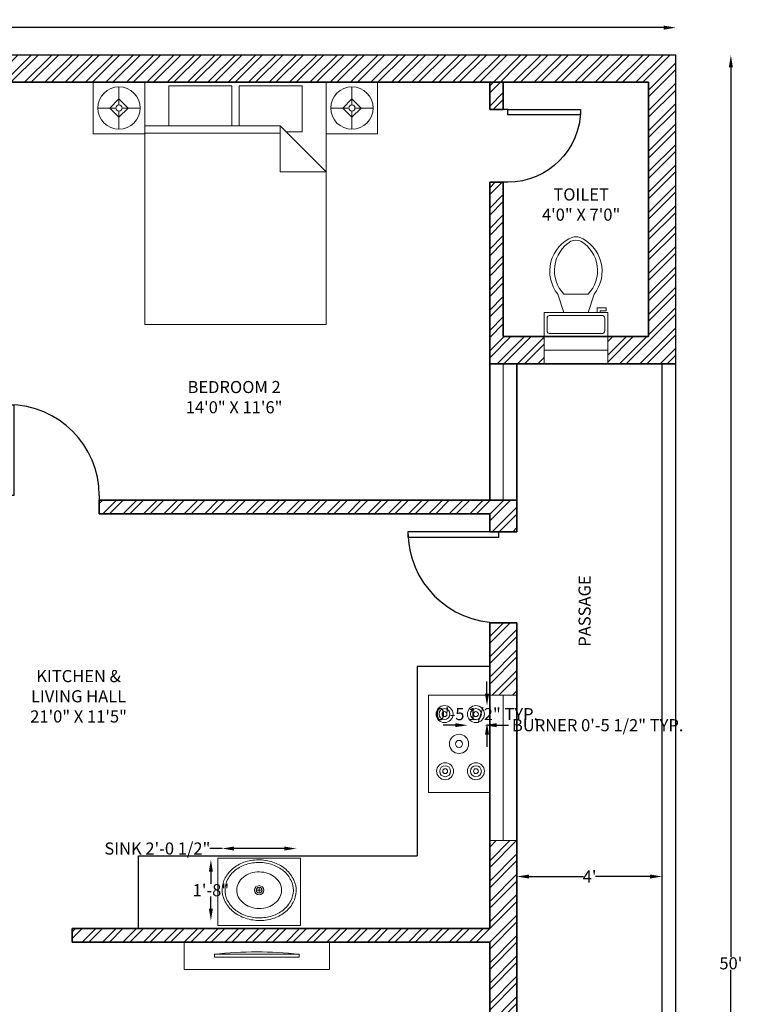
# Model space of a CAD drawing. Units: inches. Extents: x 0 to 478, y -33 to 633.
# Tile 4 of 4: x 239 to 478, y 286 to 612. Entities that reach past the tile are written whole.
import ezdxf

# ---------------------------------------------------------------- set-up
doc = ezdxf.new("R2010")
doc.units = ezdxf.units.IN
for name, color, linetype, lineweight in [('A-ANNO-DIMS', 2, 'Continuous', 18), ('A-AREA-IDEN', 7, 'Continuous', 18), ('A-DOOR', 3, 'Continuous', 25), ('A-EQPM', 8, 'Continuous', 18), ('A-FLOR-CASE', 8, 'Continuous', 25), ('A-FLOR-FIXT', 9, 'Continuous', 18), ('A-FURN', 8, 'Continuous', 18), ('A-GLAZ', 4, 'Continuous', 18), ('A-WALL', 7, 'Continuous', 35), ('A-WALL-PATT', 252, 'Continuous', 13), ('C-PROP', 7, 'Continuous', 30)]:
    doc.layers.add(name, color=color, linetype=linetype, lineweight=lineweight)
doc.styles.get("Standard").update_dxf_attribs({"font": 'arial.ttf'})
doc.dimstyles.get("Standard").update_dxf_attribs({"dimtxt": 4, "dimasz": 4, "dimexe": 0.18, "dimexo": 0.0625, "dimgap": 0.09, "dimtad": 0, "dimtih": 1, "dimtoh": 1, "dimdec": 1, "dimzin": 0, "dimdsep": 46, "dimlunit": 3, "dimtxsty": 'Standard', "dimcen": 0.09, "dimse1": 1, "dimse2": 1, "dimadec": 0, "dimazin": 0, "dimtfac": 1, "dimtdec": 1, "dimtofl": 0, "dimtmove": 0, "dimatfit": 3, "dimfxl": 1, "dimtolj": 1, "dimtzin": 0, "dimarcsym": 0})

# ---------------------------------------------------------------- blocks, each defined once
blk = doc.blocks.new('Sink - Oval top')
for p, q in [((-1, 0), (1, 0)), ((0, 1), (0, -1))]:
    blk.add_line(p, q)
for points in [[(-12.23, 0.39, 0.117634), (-11.46, -3.36, 0.104469), (-8.88, -6.8, 0.090016), (-5.08, -9.07, 0.08192), (-0.32, -10.02, 0.08192), (4.49, -9.38, 0.090016), (8.42, -7.36, 0.104469), (11.22, -4.09, 0.117634), (12.23, -0.39, 0.117634), (11.46, 3.36, 0.104469), (8.88, 6.8, 0.090016), (5.08, 9.07, 0.08192), (0.32, 10.02, 0.08192), (-4.49, 9.38, 0.090016), (-8.42, 7.36, 0.104469), (-11.22, 4.09, 0.117634)], [(-11.29, 0.16, 0.118622), (-10.52, -3.25, 0.104678), (-8.07, -6.36, 0.089562), (-4.54, -8.37, 0.081185), (-0.13, -9.15, 0.081185), (4.3, -8.49, 0.089562), (7.89, -6.58, 0.104678), (10.42, -3.55, 0.118622), (11.29, -0.16, 0.118622), (10.52, 3.25, 0.104678), (8.07, 6.36, 0.089562), (4.54, 8.37, 0.081185), (0.13, 9.15, 0.081185), (-4.3, 8.49, 0.089562), (-7.89, 6.58, 0.104678), (-10.42, 3.55, 0.118622)], [(-7.42, 0.08, 0.118283), (-6.91, -2.17, 0.104607), (-5.29, -4.21, 0.089718), (-2.97, -5.53, 0.081436), (-0.07, -6.04, 0.081436), (2.84, -5.59, 0.089718), (5.2, -4.33, 0.104607), (6.86, -2.32, 0.118283), (7.42, -0.08, 0.118283), (6.91, 2.17, 0.104607), (5.29, 4.21, 0.089718), (2.97, 5.53, 0.081436), (0.07, 6.04, 0.081436), (-2.84, 5.59, 0.089718), (-5.2, 4.33, 0.104607), (-6.86, 2.32, 0.118283)]]:
    blk.add_lwpolyline(points, format="xyb", close=True)
for radius in [1.5, 1]:
    blk.add_circle((0, 0), radius)
blk = doc.blocks.new('Bed - Queen')
for p, q in [((0, -80.00003), (0, 0)), ((0, 0), (59.99999, 0)), ((59.99999, 0), (59.99999, -80.00003)), ((7.99999, -1.2), (28.79998, -1.2)), ((7.99999, -14.4), (7.99999, -1.2)), ((28.79998, -1.2), (28.79998, -14.4)), ((31.19999, -1.2), (51.99999, -1.2)), ((31.19999, -14.4), (31.19999, -1.2)), ((51.99999, -1.2), (51.99999, -16.4)), ((0, -14.4), (44.8, -14.4)), ((59.99999, -29.6), (44.8, -14.4)), ((44.8, -14.4), (44.8, -29.6)), ((44.8, -16.8), (0, -16.8)), ((51.99999, -16.4), (46.79936, -16.4)), ((44.8, -29.6), (59.99999, -29.6)), ((59.99999, -80.00003), (0, -80.00003))]:
    blk.add_line(p, q)
blk = doc.blocks.new('Toilet - top')
for p, q in [((9.5, -6), (9.5, -2)), ((-10, -8.5), (-8, -8.5)), ((-10, -9.5), (-10, -8.5)), ((-7, -9.5), (-10, -9.5)), ((-8, -8.5), (-8, -8)), ((-7, -8), (-7, -9.5)), ((-4, -8), (-6, -14)), ((4, -8), (6, -14)), ((4, -14), (-4, -14))]:
    blk.add_line(p, q)
blk.add_lwpolyline([(10.5, -8), (10.5, 0), (-10.5, 0), (-10.5, -8)], close=True)
for points in [[(-9.5, -2), (-9.5, -6)], [(8.5, -1), (-8.5, -1)], [(-8.5, -7), (8.5, -7)]]:
    blk.add_lwpolyline(points)
for centre, radius, start, end in [((-8.62, -1.88), 0.884, 81.8699, 188.1301), ((8.62, -1.88), 0.884, 351.8699, 98.1301), ((-8.62, -6.12), 0.884, 171.8699, 278.1301), ((8.62, -6.12), 0.884, 261.8699, 8.1301), ((3.52, -21.58), 12.17, 141.4691, 247.9714), ((4.2, -21.82), 11.33, 136.3677, 238.9468), ((-3.52, -21.58), 12.17, 292.0284, 38.5307), ((-4.2, -21.82), 11.33, 301.053, 43.6321), ((0, -27.88), 4, 245.7318, 294.2682), ((0, -29), 4, 254.8605, 285.1395)]:
    blk.add_arc(centre, radius, start, end)
blk = doc.blocks.new('*U11')
for p, q in [((0, 0), (0, -6)), ((30, 0), (30, -6))]:
    blk.add_line(p, q)
blk.add_lwpolyline([(0, 0), (0, 30), (1.75, 30), (1.75, 0)], close=True)
blk.add_arc((0, 0), 30, 0, 90)
blk = doc.blocks.new('*U14')
for p, q in [((-24, 0), (-24, -6)), ((0, 0), (0, -6))]:
    blk.add_line(p, q)
blk.add_lwpolyline([(0, 0), (0, 24), (-1.75, 24), (-1.75, 0)], close=True)
blk.add_arc((0, 0), 24, 90, 180)
blk = doc.blocks.new('*U15')
for p, q in [((-30, 0), (-30, -6)), ((0, 0), (0, -6))]:
    blk.add_line(p, q)
blk.add_lwpolyline([(0, 0), (0, 30), (-1.75, 30), (-1.75, 0)], close=True)
blk.add_arc((0, 0), 30, 90, 180)
blk = doc.blocks.new('*D23')
at = {"layer": 'A-ANNO-DIMS', "color": 0, "lineweight": -2, "transparency": 16777216}
for p, q in [((407.5, 328.66), (425.49, 328.66)), ((447.5, 328.66), (429.51, 328.66))]:
    blk.add_line(p, q, dxfattribs=at)
at = {"layer": 'A-ANNO-DIMS', "color": 0, "transparency": 16777216}
for points in [[(407.5, 329.32), (407.5, 327.99), (403.5, 328.66)], [(447.5, 329.32), (447.5, 327.99), (451.5, 328.66)]]:
    blk.add_solid(points, dxfattribs=at)
at = {"layer": 'Defpoints', "color": 0, "transparency": 16777216}
for p in [(403.5, 340.53), (451.5, 340.53), (451.5, 328.66)]:
    blk.add_point(p, dxfattribs=at)
at = {"layer": 'A-ANNO-DIMS', "color": 0, "transparency": 16777216, "insert": (427.5, 328.66), "char_height": 4, "attachment_point": 5}
blk.add_mtext("\\A1;4'", dxfattribs=at)
blk = doc.blocks.new('*D24')
at = {"layer": 'A-ANNO-DIMS', "color": 0, "lineweight": -2, "transparency": 16777216}
for p, q in [((474.18, 596), (474.18, 302.13)), ((474.18, 4), (474.18, 297.87))]:
    blk.add_line(p, q, dxfattribs=at)
at = {"layer": 'A-ANNO-DIMS', "color": 0, "transparency": 16777216}
for points in [[(473.51, 596), (474.84, 596), (474.18, 600)], [(473.51, 4), (474.84, 4), (474.18, 0)]]:
    blk.add_solid(points, dxfattribs=at)
at = {"layer": 'Defpoints', "color": 0, "transparency": 16777216}
for p in [(456, 600), (474.18, 600), (456, 0)]:
    blk.add_point(p, dxfattribs=at)
at = {"layer": 'A-ANNO-DIMS', "color": 0, "transparency": 16777216, "insert": (474.18, 300), "char_height": 4, "attachment_point": 5}
blk.add_mtext("\\A1;50'", dxfattribs=at)
blk = doc.blocks.new('*D25')
at = {"layer": 'A-ANNO-DIMS', "color": 0, "lineweight": -2, "transparency": 16777216}
for p, q in [((4, 609.06), (224.52, 609.06)), ((452, 609.06), (231.48, 609.06))]:
    blk.add_line(p, q, dxfattribs=at)
at = {"layer": 'A-ANNO-DIMS', "color": 0, "transparency": 16777216}
for points in [[(4, 609.73), (4, 608.4), (0, 609.06)], [(452, 609.73), (452, 608.4), (456, 609.06)]]:
    blk.add_solid(points, dxfattribs=at)
at = {"layer": 'Defpoints', "color": 0, "transparency": 16777216}
for p in [(0, 609.06), (0, 600), (456, 600)]:
    blk.add_point(p, dxfattribs=at)
at = {"layer": 'A-ANNO-DIMS', "color": 0, "transparency": 16777216, "insert": (228, 609.06), "char_height": 4, "attachment_point": 5}
blk.add_mtext("\\A1;38'", dxfattribs=at)
blk = doc.blocks.new('WIN-48IN')
for p, q in [((0, 48), (9, 48)), ((4.5, 48), (4.5, 0)), ((0, 0), (9, 0))]:
    blk.add_line(p, q)
blk = doc.blocks.new('WIN-21IN')
for p, q in [((0, 9), (0, 0)), ((21, 9), (21, 0)), ((0, 4.5), (21, 4.5))]:
    blk.add_line(p, q)
blk = doc.blocks.new('Lamp - Table')
for p, q in [((0, 7), (0, 1)), ((-1, 0), (-7, 0)), ((0, 3), (-3, 0)), ((-3, 0), (0, -3)), ((3, 0), (0, 3)), ((0, -3), (3, 0)), ((1, 0), (7, 0)), ((0, -1), (0, -7))]:
    blk.add_line(p, q)
for radius in [7, 1]:
    blk.add_circle((0, 0), radius)
blk = doc.blocks.new('END-TABLE-WITH-LAMP')
blk.add_lwpolyline([(-8.49, 8.49), (-8.49, -8.49), (8.49, -8.49), (8.49, 8.49)], close=True)
blk.add_blockref('Lamp - Table', (0, 0))
blk = doc.blocks.new('COOKTOP-BURNER')
for radius in [2.81, 1.81, 0.809]:
    blk.add_circle((0, 0), radius)
blk = doc.blocks.new('*D36')
at = {"layer": 'A-ANNO-DIMS', "color": 0, "lineweight": -2, "transparency": 16777216}
for p, q in [((383.14, 378.65), (379.14, 378.65)), ((396.76, 378.65), (400.76, 378.65))]:
    blk.add_line(p, q, dxfattribs=at)
at = {"layer": 'A-ANNO-DIMS', "color": 0, "transparency": 16777216}
for points in [[(383.14, 379.32), (383.14, 377.99), (387.14, 378.65)], [(396.76, 379.32), (396.76, 377.99), (392.76, 378.65)]]:
    blk.add_solid(points, dxfattribs=at)
at = {"layer": 'Defpoints', "color": 0, "transparency": 16777216}
for p in [(387.14, 379.5), (392.76, 379.5), (392.76, 378.65)]:
    blk.add_point(p, dxfattribs=at)
at = {"layer": 'A-ANNO-DIMS', "color": 0, "transparency": 16777216, "insert": (430.19, 378.65), "char_height": 4, "attachment_point": 5}
blk.add_mtext('\\A1;BURNER 0\'-5 1/2" TYP.', dxfattribs=at)
blk = doc.blocks.new('*D37')
at = {"layer": 'A-ANNO-DIMS', "color": 0, "lineweight": -2, "transparency": 16777216}
for p, q in [((393.6, 389.11), (393.6, 393.11)), ((393.6, 375.5), (393.6, 371.5))]:
    blk.add_line(p, q, dxfattribs=at)
at = {"layer": 'A-ANNO-DIMS', "color": 0, "transparency": 16777216}
for points in [[(392.94, 389.11), (394.27, 389.11), (393.6, 385.11)], [(392.94, 375.5), (394.27, 375.5), (393.6, 379.5)]]:
    blk.add_solid(points, dxfattribs=at)
at = {"layer": 'Defpoints', "color": 0, "transparency": 16777216}
for p in [(392.76, 385.11), (393.6, 385.11), (392.76, 379.5)]:
    blk.add_point(p, dxfattribs=at)
at = {"layer": 'A-ANNO-DIMS', "color": 0, "transparency": 16777216, "insert": (393.6, 382.31), "char_height": 4, "attachment_point": 5}
blk.add_mtext('\\A1;0\'-5 1/2" TYP.', dxfattribs=at)
blk = doc.blocks.new('*D52')
at = {"layer": 'A-ANNO-DIMS', "color": 0, "lineweight": -2, "transparency": 16777216}
for p, q in [((306.06, 337.91), (302.06, 337.91)), ((326.61, 337.91), (310.06, 337.91))]:
    blk.add_line(p, q, dxfattribs=at)
at = {"layer": 'A-ANNO-DIMS', "color": 0, "transparency": 16777216}
for points in [[(310.06, 338.57), (310.06, 337.24), (306.06, 337.91)], [(326.61, 338.57), (326.61, 337.24), (330.61, 337.91)]]:
    blk.add_solid(points, dxfattribs=at)
at = {"layer": 'Defpoints', "color": 0, "transparency": 16777216}
for p in [(306.06, 337.91), (306.06, 334.22), (330.61, 334.22)]:
    blk.add_point(p, dxfattribs=at)
at = {"layer": 'A-ANNO-DIMS', "color": 0, "transparency": 16777216, "insert": (284.7, 337.91), "char_height": 4, "attachment_point": 5}
blk.add_mtext('\\A1;SINK 2\'-0 1/2"', dxfattribs=at)
blk = doc.blocks.new('*D53')
at = {"layer": 'A-ANNO-DIMS', "color": 0, "lineweight": -2, "transparency": 16777216}
for p, q in [((302.38, 330.22), (302.38, 326.29)), ((302.38, 318.09), (302.38, 322.02))]:
    blk.add_line(p, q, dxfattribs=at)
at = {"layer": 'A-ANNO-DIMS', "color": 0, "transparency": 16777216}
for points in [[(301.71, 330.22), (303.04, 330.22), (302.38, 334.22)], [(301.71, 318.09), (303.04, 318.09), (302.38, 314.09)]]:
    blk.add_solid(points, dxfattribs=at)
at = {"layer": 'Defpoints', "color": 0, "transparency": 16777216}
for p in [(306.06, 334.22), (302.38, 314.09), (306.06, 314.09)]:
    blk.add_point(p, dxfattribs=at)
at = {"layer": 'A-ANNO-DIMS', "color": 0, "transparency": 16777216, "insert": (302.38, 324.15), "char_height": 4, "attachment_point": 5}
blk.add_mtext('\\A1;1\'-8"', dxfattribs=at)
blk = doc.blocks.new('*D57')
at = {"layer": 'A-ANNO-DIMS', "color": 0, "lineweight": -2, "transparency": 16777216}
for p, q in [((239.5, -30.8), (245.06, -30.8)), ((261.5, -30.8), (255.94, -30.8))]:
    blk.add_line(p, q, dxfattribs=at)
at = {"layer": 'A-ANNO-DIMS', "color": 0, "transparency": 16777216}
for points in [[(239.5, -30.13), (239.5, -31.47), (235.5, -30.8)], [(261.5, -30.13), (261.5, -31.47), (265.5, -30.8)]]:
    blk.add_solid(points, dxfattribs=at)
at = {"layer": 'Defpoints', "color": 0, "transparency": 16777216}
for p in [(235.5, 448.5), (265.5, 448.5), (265.5, -30.8)]:
    blk.add_point(p, dxfattribs=at)
at = {"layer": 'A-ANNO-DIMS', "color": 0, "transparency": 16777216, "insert": (250.5, -30.8), "char_height": 4, "attachment_point": 5}
blk.add_mtext('\\A1;2\'-6"', dxfattribs=at)

msp = doc.modelspace()

# ---------------------------------------------------------------- hatches: boundary and pattern name
at = {"layer": 'A-WALL-PATT'}
h = msp.add_hatch(dxfattribs=at)
h.set_pattern_fill('ANSI32', color=256, scale=0.5)
h.paths.add_polyline_path([(456, 600), (45, 600), (45, 547.04), (54, 547.04), (54, 591), (447, 591), (447, 507), (433.5, 507), (433.5, 498), (456, 498)])
h.paths.add_polyline_path([(54, 499.04), (45, 499.04), (45, 429), (54, 429)])
h.paths.add_polyline_path([(235.5, 453), (226.5, 453), (226.5, 591), (222, 591), (222, 453), (213, 453), (213, 448.5), (235.5, 448.5)])
h.paths.add_polyline_path([(105, 453), (54, 453), (54, 448.5), (105, 448.5)], flags=17)
h.paths.add_polyline_path([(183, 453), (129, 453), (129, 448.5), (138, 448.5), (138, 388.5), (54, 388.5), (54, 384), (138, 384), (138, 324), (129, 324), (129, 319.5), (192, 319.5), (192, 310.5), (196.5, 310.5), (196.5, 324), (142.5, 324), (142.5, 448.5), (183, 448.5)])
h.paths.add_polyline_path([(403.5, 453), (265.5, 453), (265.5, 448.5), (394.5, 448.5), (394.5, 442.5), (397.5, 442.5), (403.5, 442.5)])
h.paths.add_polyline_path([(412.5, 507), (399, 507), (399, 558), (394.5, 558), (394.5, 498), (412.5, 498)], flags=17)
h.paths.add_polyline_path([(399, 591), (394.5, 591), (394.5, 582), (399, 582)], flags=17)
h.paths.add_polyline_path([(54, 408), (45, 408), (45, 364.5), (54, 364.5)])
h.paths.add_polyline_path([(54, 343.5), (45, 343.5), (45, 275.82), (54, 275.82), (54, 319.5)])
h.paths.add_polyline_path([(105, 324), (54, 324), (54, 319.5), (105, 319.5)], flags=17)
h.paths.add_polyline_path([(403.5, 412.5), (397.5, 412.5), (394.5, 412.5), (394.5, 388.53), (403.5, 388.53)])
h.paths.add_polyline_path([(403.5, 340.53), (394.5, 340.53), (394.5, 311.5), (256.5, 311.5), (256.5, 307), (394.5, 307), (394.5, 255.85), (403.5, 255.85)])
h.paths.add_polyline_path([(54, 216.47), (54, 227.82), (45, 227.82), (45, 190.5), (95.47, 190.5), (95.47, 199.5), (70.97, 199.5), (54, 199.5)])
h.paths.add_polyline_path([(196.5, 280.5), (192, 280.5), (192, 199.5), (143.47, 199.5), (143.47, 190.5), (187.5, 190.5), (187.5, 188.75), (193.5, 188.75), (196.5, 188.75)])
h.paths.add_polyline_path([(403.5, 207.85), (394.5, 207.85), (394.5, 126.5), (403.5, 126.5)])
h.paths.add_polyline_path([(403.5, 78.5), (394.5, 78.5), (394.5, 63), (265.7, 63), (265.7, 54), (403.5, 54)])
h.paths.add_polyline_path([(394.5, 151), (313.7, 151), (313.7, 142), (394.5, 142)])
h.paths.add_polyline_path([(265.7, 151), (196.5, 151), (196.5, 152.75), (193.5, 152.75), (187.5, 152.75), (187.5, 142), (265.7, 142)])

# ---------------------------------------------------------------- linework, layer by layer
at = {"layer": 'A-EQPM'}
for points in [[(394.5, 388.53), (394.5, 356.41), (374.24, 356.41), (374.24, 388.53)], [(293.52, 307), (341.52, 307), (341.52, 298), (293.52, 298)], [(303.52, 303), (331.52, 303), (331.52, 302), (303.52, 302)]]:
    msp.add_lwpolyline(points, close=True, dxfattribs=at)
for radius in [3.17, 1.17]:
    msp.add_circle((384.37, 372.47), radius, dxfattribs=at)
msp.add_arc((317.52, 172.09), 131.66, 83.8959, 96.1041, dxfattribs=at)
at = {"layer": 'A-FLOR-CASE'}
for p, q in [((394.5, 398), (370.5, 398)), ((370.5, 398), (370.5, 335.5)), ((278.44, 311.5), (278.44, 335.5)), ((278.44, 335.5), (370.5, 335.5))]:
    msp.add_line(p, q, dxfattribs=at)
at = {"layer": 'A-FLOR-FIXT'}
msp.add_lwpolyline([(304.64, 312.44), (304.64, 334.7), (332.02, 334.7), (332.02, 312.44)], close=True, dxfattribs=at)
at = {"layer": 'A-GLAZ'}
msp.add_line((399, 498), (399, 453), dxfattribs=at)
at = {"layer": 'A-WALL'}
for p, q in [((447, 591), (54, 591)), ((394.5, 591), (394.5, 582)), ((399, 591), (399, 582)), ((447, 507), (447, 591)), ((394.5, 582), (399, 582)), ((394.5, 558), (394.5, 498)), ((394.5, 558), (399, 558)), ((399, 558), (399, 507)), ((399, 507), (447, 507)), ((394.5, 453), (394.5, 498)), ((394.5, 498), (456, 498)), ((403.5, 442.5), (403.5, 498)), ((456, 498), (408, 498)), ((403.5, 453), (265.5, 453)), ((265.5, 453), (265.5, 448.5)), ((394.5, 448.5), (265.5, 448.5)), ((394.5, 442.5), (394.5, 448.5)), ((394.5, 442.5), (403.5, 442.5)), ((394.5, 311.5), (394.5, 412.5)), ((394.5, 412.5), (403.5, 412.5)), ((403.5, 54), (403.5, 412.5)), ((394.5, 311.5), (256.5, 311.5)), ((256.5, 311.5), (256.5, 307)), ((394.5, 307), (256.5, 307)), ((394.5, 63), (394.5, 307))]:
    msp.add_line(p, q, dxfattribs=at)
at = {"layer": 'C-PROP'}
for p, q in [((456, 600), (0, 600)), ((456, 0), (456, 600)), ((451.5, 8), (451.5, 498))]:
    msp.add_line(p, q, dxfattribs=at)

# ---------------------------------------------------------------- block references
at = {"layer": 'A-DOOR', "xscale": -1, "rotation": 270}
msp.add_blockref('*U14', (400.5, 582), dxfattribs=at)
at = {"layer": 'A-DOOR'}
msp.add_blockref('*U11', (235.5, 454.5), dxfattribs=at)
at = {"layer": 'A-DOOR', "rotation": 90.00000000000003}
msp.add_blockref('*U15', (397.5, 442.5), dxfattribs=at)
at = {"layer": 'A-EQPM'}
for p in [(379.57, 382.31), (389.95, 382.31), (379.78, 363.45), (389.95, 363.45)]:
    msp.add_blockref('COOKTOP-BURNER', p, dxfattribs=at)
at = {"layer": 'A-FLOR-FIXT', "rotation": 180}
for name, p in [('Toilet - top', (423, 507)), ('Sink - Oval top', (318.33, 324.15))]:
    msp.add_blockref(name, p, dxfattribs=at)
at = {"layer": 'A-FURN'}
for name, p in [('END-TABLE-WITH-LAMP', (272.01, 582.51)), ('Bed - Queen', (280.5, 591))]:
    msp.add_blockref(name, p, dxfattribs=at)
at = {"layer": 'A-FURN', "extrusion": (0, 0, -1), "zscale": -1}
msp.add_blockref('END-TABLE-WITH-LAMP', (-348.99, 582.51), dxfattribs=at)
at = {"layer": 'A-GLAZ'}
for name, p in [('WIN-21IN', (412.5, 498)), ('WIN-48IN', (394.5, 340.53))]:
    msp.add_blockref(name, p, dxfattribs=at)

# ---------------------------------------------------------------- texts
at = {"layer": 'A-AREA-IDEN', "ltscale": 0.5, "char_height": 4, "attachment_point": 1}
for s, insert in [('\\pxqc;TOILET\\P4\'0" X 7\'0"', (405.84, 555.96)), ('\\pxqc;BEDROOM 2\\P14\'0" X 11\'6"', (291.18, 492.34)), ('\\pxqc;KITCHEN & LIVING HALL\\P21\'0" X 11\'5"', (239.79, 396.87))]:
    msp.add_mtext_dynamic_manual_height_columns(s, width=37.7397, gutter_width=12.5, heights=[0], dxfattribs=dict(at, insert=insert))
at = {"layer": 'A-AREA-IDEN', "ltscale": 0.5, "insert": (423.86, 397.49), "char_height": 4, "attachment_point": 1, "rotation": 90}
msp.add_mtext_dynamic_manual_height_columns('\\pxqc;PASSAGE', width=37.7397, gutter_width=12.5, heights=[0], dxfattribs=at)

# ---------------------------------------------------------------- dimensions: what is measured, and where the dimension line sits
at = {"layer": 'A-ANNO-DIMS'}
for base, p1, p2, override, picture, middle in [((0, 609.06), (456, 600), (0, 600), {"dimclrd": 0, "dimclre": 0, "dimclrt": 0}, '*D25', (228, 609.06)), ((265.5, -30.8), (235.5, 448.5), (265.5, 448.5), {"dimdec": 1, "dimlfac": 1, "dimrnd": 0, "dimzin": 1, "dimdsep": 46, "dimlunit": 4, "dimfrac": 2}, '*D57', (250.5, -30.8)), ((451.5, 328.66), (403.5, 340.53), (451.5, 340.53), {"dimclrd": 0, "dimclre": 0, "dimclrt": 0}, '*D23', (427.5, 328.66))]:
    dim = msp.add_linear_dim(base=base, p1=p1, p2=p2, dimstyle='Standard', override=override, dxfattribs=at)
    dim.commit()
    dim.dimension.update_dxf_attribs({"geometry": picture, "text_midpoint": middle})
for base, p1, p2, angle, override, picture, middle in [((474.18, 600), (456, 0), (456, 600), 90, {"dimclrd": 0, "dimclre": 0, "dimclrt": 0}, '*D24', (474.18, 300)), ((302.38, 314.09), (306.06, 334.22), (306.06, 314.09), 270, {"dimdec": 1, "dimlfac": 1, "dimrnd": 0, "dimzin": 1, "dimdsep": 46, "dimlunit": 4, "dimfrac": 2}, '*D53', (302.38, 324.15))]:
    dim = msp.add_linear_dim(base=base, p1=p1, p2=p2, angle=angle, dimstyle='Standard', override=override, dxfattribs=at)
    dim.commit()
    dim.dimension.update_dxf_attribs({"geometry": picture, "text_midpoint": middle})
for base, p1, p2, angle, text, picture, middle in [((393.6, 385.11), (392.76, 379.5), (392.76, 385.11), 90, '<> TYP.', '*D37', (393.6, 382.31)), ((306.0586, 337.9057), (330.6095, 334.223), (306.0586, 334.223), 180, 'SINK <>', '*D52', (284.704, 337.9057))]:
    dim = msp.add_linear_dim(base=base, p1=p1, p2=p2, angle=angle, text=text, dimstyle='Standard', override={"dimdec": 1, "dimlfac": 1, "dimrnd": 0, "dimzin": 1, "dimdsep": 46, "dimlunit": 4, "dimfrac": 2}, dxfattribs=at)
    dim.commit()
    dim.dimension.update_dxf_attribs({"geometry": picture, "text_midpoint": middle})
dim = msp.add_linear_dim(base=(392.76, 378.65), p1=(387.14, 379.5), p2=(392.76, 379.5), text='BURNER <> TYP.', dimstyle='Standard', override={"dimdec": 1, "dimlfac": 1, "dimrnd": 0, "dimzin": 1, "dimdsep": 46, "dimlunit": 4, "dimfrac": 2}, dxfattribs=at)
dim.commit()
dim.dimension.update_dxf_attribs({"geometry": '*D36', "text_midpoint": (430.19, 378.65)})

doc.saveas('drawing.dxf')
